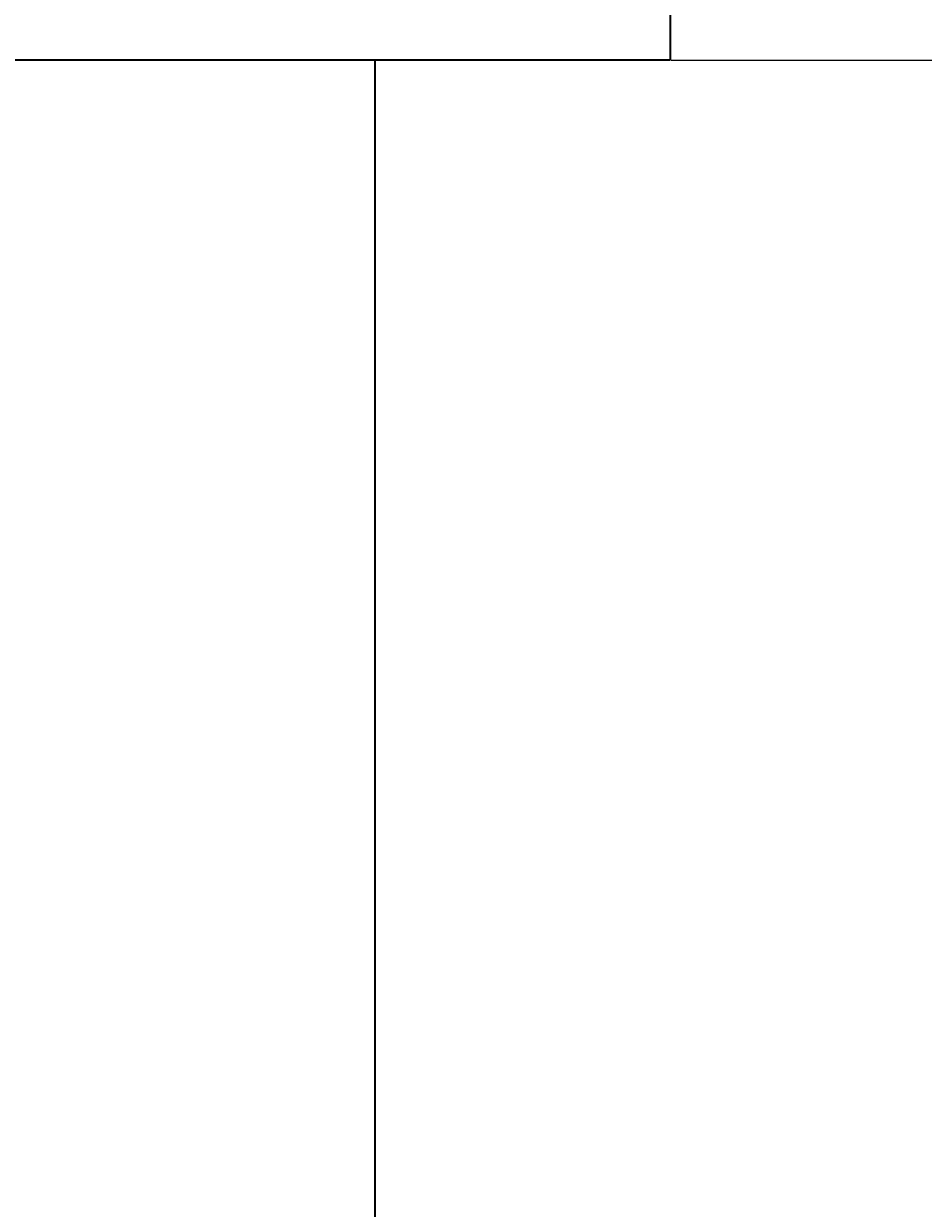
# Model space of a CAD drawing. Units: inches. Extents: x -13 to 809, y 112 to 656.
# Tile 53 of 55: x 593 to 665, y 467 to 561. Entities that reach past the tile are written whole.
import ezdxf

# ---------------------------------------------------------------- set-up
doc = ezdxf.new("R2010")
doc.units = ezdxf.units.IN
doc.header["$MEASUREMENT"] = 0
doc.layers.add('A-ANNO-DIMS', color=2, linetype='Continuous', lineweight=18)
doc.layers.add('A-ELEV', color=7, linetype='Continuous', lineweight=35)
doc.styles.get("Standard").update_dxf_attribs({"font": 'arial.ttf'})
doc.dimstyles.get("Standard").update_dxf_attribs({"dimtxt": 0.625, "dimasz": 0.18, "dimexe": 0.18, "dimexo": 0.0625, "dimgap": 0.09, "dimtad": 0, "dimtih": 1, "dimtoh": 1, "dimdec": 4, "dimzin": 0, "dimdsep": 46, "dimlunit": 4, "dimtxsty": 'Standard', "dimcen": 0.09, "dimadec": 0, "dimazin": 0, "dimtfac": 1, "dimtdec": 4, "dimtofl": 0, "dimtmove": 0, "dimatfit": 3, "dimfxl": 1, "dimtolj": 1, "dimtzin": 0, "dimarcsym": 0})

# ---------------------------------------------------------------- blocks, each defined once
blk = doc.blocks.new('*D29')
at = {"layer": 'A-ANNO-DIMS', "color": 0, "lineweight": -2, "transparency": 16777216}
for p, q in [((591.008, 558.582), (591.008, 655.963)), ((591.188, 655.783), (605.472, 655.783)), ((620.828, 655.783), (606.544, 655.783)), ((621.008, 617.845), (621.008, 655.963))]:
    blk.add_line(p, q, dxfattribs=at)
at = {"layer": 'A-ANNO-DIMS', "color": 0, "transparency": 16777216}
for points in [[(591.188, 655.813), (591.188, 655.753), (591.008, 655.783)], [(620.828, 655.813), (620.828, 655.753), (621.008, 655.783)]]:
    blk.add_solid(points, dxfattribs=at)
at = {"layer": 'Defpoints', "color": 0, "transparency": 16777216}
for p in [(621.008, 655.783), (621.008, 617.783), (591.008, 558.52)]:
    blk.add_point(p, dxfattribs=at)
at = {"layer": 'A-ANNO-DIMS', "color": 0, "transparency": 16777216, "insert": (606.008, 655.783), "char_height": 0.625, "attachment_point": 5}
blk.add_mtext('\\A1;30', dxfattribs=at)
blk = doc.blocks.new('*D31')
at = {"layer": 'A-ANNO-DIMS', "color": 0, "lineweight": -2, "transparency": 16777216}
for p, q in [((621.071, 617.783), (807.769, 617.783)), ((807.589, 617.603), (807.589, 384.561)), ((807.589, 150.7), (807.589, 383.742)), ((621.071, 150.52), (807.769, 150.52))]:
    blk.add_line(p, q, dxfattribs=at)
at = {"layer": 'A-ANNO-DIMS', "color": 0, "transparency": 16777216}
for points in [[(807.559, 617.603), (807.619, 617.603), (807.589, 617.783)], [(807.559, 150.7), (807.619, 150.7), (807.589, 150.52)]]:
    blk.add_solid(points, dxfattribs=at)
at = {"layer": 'Defpoints', "color": 0, "transparency": 16777216}
for p in [(621.008, 617.783), (807.589, 617.783), (621.008, 150.52)]:
    blk.add_point(p, dxfattribs=at)
at = {"layer": 'A-ANNO-DIMS', "color": 0, "transparency": 16777216, "insert": (807.589, 384.151), "char_height": 0.625, "attachment_point": 5}
blk.add_mtext('\\A1;467.3', dxfattribs=at)
blk = doc.blocks.new('*D38')
at = {"layer": 'A-ANNO-DIMS', "color": 0, "lineweight": -2, "transparency": 16777216}
for p, q in [((644.685, 569.241), (807.769, 569.241)), ((807.589, 569.061), (807.589, 564.29)), ((807.589, 558.7), (807.589, 563.472)), ((644.685, 558.52), (807.769, 558.52))]:
    blk.add_line(p, q, dxfattribs=at)
at = {"layer": 'A-ANNO-DIMS', "color": 0, "transparency": 16777216}
for points in [[(807.559, 569.061), (807.619, 569.061), (807.589, 569.241)], [(807.559, 558.7), (807.619, 558.7), (807.589, 558.52)]]:
    blk.add_solid(points, dxfattribs=at)
at = {"layer": 'Defpoints', "color": 0, "transparency": 16777216}
for p in [(644.622, 569.241), (807.589, 569.241), (644.622, 558.52)]:
    blk.add_point(p, dxfattribs=at)
at = {"layer": 'A-ANNO-DIMS', "color": 0, "transparency": 16777216, "insert": (807.589, 563.881), "char_height": 0.625, "attachment_point": 5}
blk.add_mtext('\\A1;10.721', dxfattribs=at)

msp = doc.modelspace()

# ---------------------------------------------------------------- linework, layer by layer
at = {"layer": 'A-ELEV'}
for p, q in [((644.6221, 569.2414), (644.6221, 558.5199)), ((644.6221, 558.5199), (591.008, 558.5199)), ((621.008, 209.8635), (621.008, 558.5199))]:
    msp.add_line(p, q, dxfattribs=at)

# ---------------------------------------------------------------- dimensions: what is measured, and where the dimension line sits
at = {"layer": 'A-ANNO-DIMS'}
dim = msp.add_linear_dim(base=(621.008, 655.7828), p1=(591.008, 558.5199), p2=(621.008, 617.7828), dimstyle='Standard', override={"dimdec": 0, "dimlfac": 1, "dimrnd": 0, "dimzin": 0, "dimdsep": 46, "dimlunit": 2}, dxfattribs=at)
dim.commit()
dim.dimension.update_dxf_attribs({"geometry": '*D29', "text_midpoint": (606.008, 655.7828)})
for base, p1, p2, override, picture, middle in [((807.5888, 617.7828), (621.008, 150.5199), (621.008, 617.7828), {"dimdec": 1, "dimlfac": 1, "dimrnd": 0, "dimzin": 0, "dimdsep": 46, "dimlunit": 2}, '*D31', (807.5888, 384.1514)), ((807.588831, 569.241385), (644.622094, 558.519894), (644.622094, 569.241385), {"dimdec": 3, "dimlfac": 1, "dimrnd": 0, "dimzin": 0, "dimdsep": 46, "dimlunit": 2}, '*D38', (807.588831, 563.88064))]:
    dim = msp.add_linear_dim(base=base, p1=p1, p2=p2, angle=90, dimstyle='Standard', override=override, dxfattribs=at)
    dim.commit()
    dim.dimension.update_dxf_attribs({"geometry": picture, "text_midpoint": middle})

doc.saveas('drawing.dxf')
